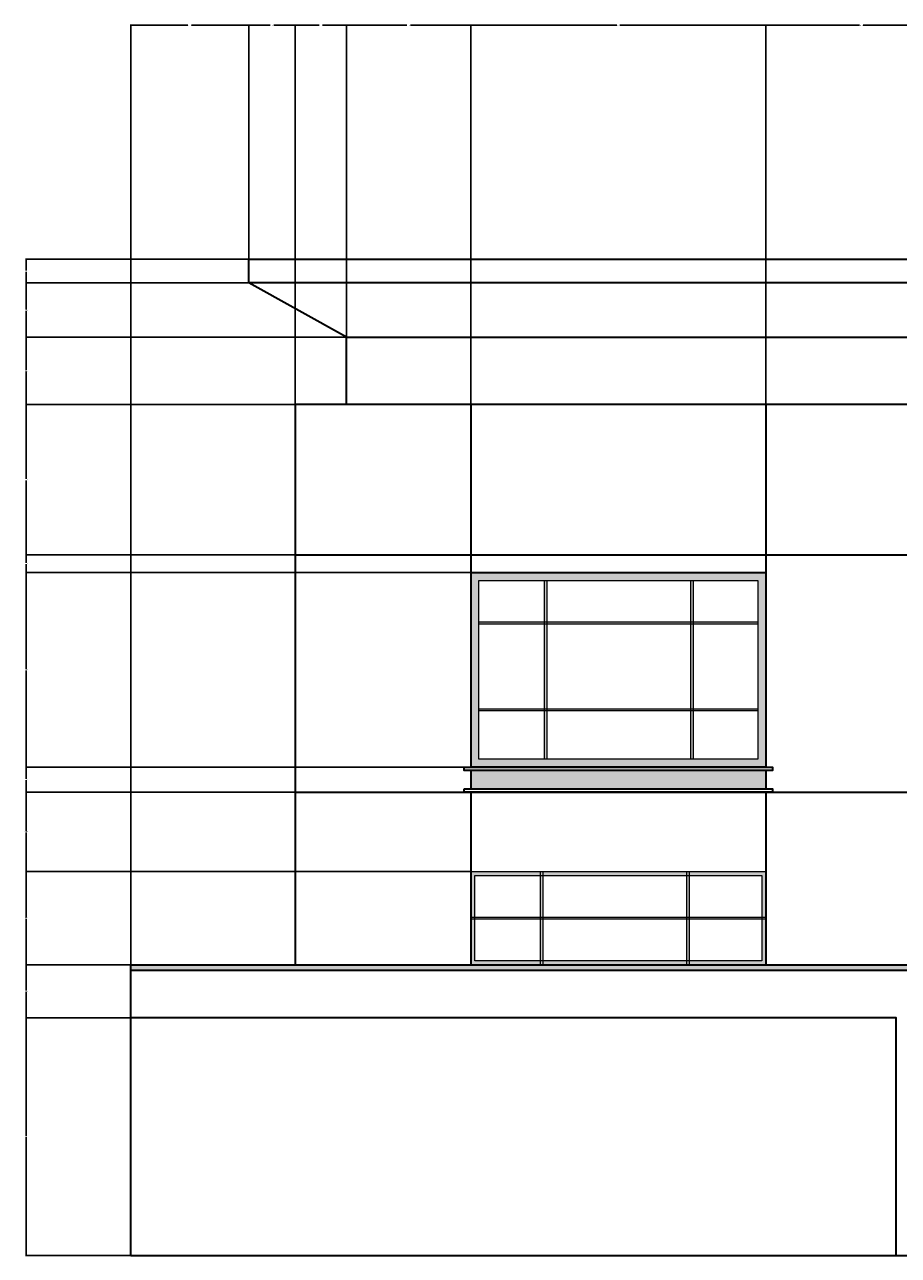
# Model space of a CAD drawing. Units: feet. Extents: x 2651 to 4047, y 949 to 1287.
# Tile 4 of 5: x 3468 to 3689, y 976 to 1287. Entities that reach past the tile are written whole.
import ezdxf

# ---------------------------------------------------------------- set-up
doc = ezdxf.new("R2010")
doc.units = ezdxf.units.FT
for name, color, linetype, lineweight in [('A-ANNO-DIMS', 2, 'Continuous', 18), ('A-ELEV', 7, 'Continuous', 35), ('A-ELEV-PATT', 8, 'Continuous', 13), ('A-GLAZ', 4, 'Continuous', 18)]:
    doc.layers.add(name, color=color, linetype=linetype, lineweight=lineweight)
doc.styles.get("Standard").update_dxf_attribs({"font": 'arial.ttf'})
doc.dimstyles.get("Standard").update_dxf_attribs({"dimtxt": 0.18, "dimasz": 0.18, "dimexe": 0.18, "dimexo": 0.0625, "dimgap": 0.09, "dimtad": 0, "dimtih": 1, "dimtoh": 1, "dimdec": 1, "dimzin": 0, "dimdsep": 46, "dimlunit": 3, "dimtxsty": 'Standard', "dimcen": 0.09, "dimadec": 0, "dimazin": 0, "dimtfac": 1, "dimtdec": 1, "dimtofl": 0, "dimtmove": 0, "dimatfit": 3, "dimfxl": 1, "dimtolj": 1, "dimtzin": 0, "dimarcsym": 0})

# ---------------------------------------------------------------- blocks, each defined once
blk = doc.blocks.new('*D25')
at = {"layer": 'A-ANNO-DIMS', "color": 0, "lineweight": -2, "transparency": 16777216}
for p, q in [((3495.28, 1049.25), (3495.28, 1287.01)), ((3495.46, 1286.83), (3509.71, 1286.83)), ((3524.89, 1286.83), (3510.64, 1286.83)), ((3525.07, 1227.71), (3525.07, 1287.01))]:
    blk.add_line(p, q, dxfattribs=at)
at = {"layer": 'A-ANNO-DIMS', "color": 0, "transparency": 16777216}
for points in [[(3495.46, 1286.86), (3495.46, 1286.8), (3495.28, 1286.83)], [(3524.89, 1286.86), (3524.89, 1286.8), (3525.07, 1286.83)]]:
    blk.add_solid(points, dxfattribs=at)
at = {"layer": 'Defpoints', "color": 0, "transparency": 16777216}
for p in [(3525.07, 1286.83), (3525.07, 1227.65), (3495.28, 1049.19)]:
    blk.add_point(p, dxfattribs=at)
at = {"layer": 'A-ANNO-DIMS', "color": 0, "transparency": 16777216, "insert": (3510.17, 1286.83), "char_height": 0.18, "attachment_point": 5}
blk.add_mtext('\\A1;29.795', dxfattribs=at)
blk = doc.blocks.new('*D26')
at = {"layer": 'A-ANNO-DIMS', "color": 0, "lineweight": -2, "transparency": 16777216}
for p, q in [((3525.07, 1227.71), (3525.07, 1287.01)), ((3525.25, 1286.83), (3530.49, 1286.83)), ((3536.64, 1286.83), (3531.4, 1286.83)), ((3536.82, 1190.93), (3536.82, 1287.01))]:
    blk.add_line(p, q, dxfattribs=at)
at = {"layer": 'A-ANNO-DIMS', "color": 0, "transparency": 16777216}
for points in [[(3525.25, 1286.86), (3525.25, 1286.8), (3525.07, 1286.83)], [(3536.64, 1286.86), (3536.64, 1286.8), (3536.82, 1286.83)]]:
    blk.add_solid(points, dxfattribs=at)
at = {"layer": 'Defpoints', "color": 0, "transparency": 16777216}
for p in [(3536.82, 1286.83), (3525.07, 1227.65), (3536.82, 1190.87)]:
    blk.add_point(p, dxfattribs=at)
at = {"layer": 'A-ANNO-DIMS', "color": 0, "transparency": 16777216, "insert": (3530.95, 1286.83), "char_height": 0.18, "attachment_point": 5}
blk.add_mtext('\\A1;11.753', dxfattribs=at)
blk = doc.blocks.new('*D27')
at = {"layer": 'A-ANNO-DIMS', "color": 0, "lineweight": -2, "transparency": 16777216}
for p, q in [((3536.82, 1190.93), (3536.82, 1287.01)), ((3537, 1286.83), (3542.92, 1286.83)), ((3549.6, 1286.83), (3543.69, 1286.83)), ((3549.78, 1208.02), (3549.78, 1287.01))]:
    blk.add_line(p, q, dxfattribs=at)
at = {"layer": 'A-ANNO-DIMS', "color": 0, "transparency": 16777216}
for points in [[(3537, 1286.86), (3537, 1286.8), (3536.82, 1286.83)], [(3549.6, 1286.86), (3549.6, 1286.8), (3549.78, 1286.83)]]:
    blk.add_solid(points, dxfattribs=at)
at = {"layer": 'Defpoints', "color": 0, "transparency": 16777216}
for p in [(3549.78, 1286.83), (3549.78, 1207.95), (3536.82, 1190.87)]:
    blk.add_point(p, dxfattribs=at)
at = {"layer": 'A-ANNO-DIMS', "color": 0, "transparency": 16777216, "insert": (3543.3, 1286.83), "char_height": 0.18, "attachment_point": 5}
blk.add_mtext('\\A1;12.96', dxfattribs=at)
blk = doc.blocks.new('*D28')
at = {"layer": 'A-ANNO-DIMS', "color": 0, "lineweight": -2, "transparency": 16777216}
for p, q in [((3549.78, 1208.02), (3549.78, 1287.01)), ((3549.96, 1286.83), (3565.05, 1286.83)), ((3581.07, 1286.83), (3565.98, 1286.83)), ((3581.25, 1190.93), (3581.25, 1287.01))]:
    blk.add_line(p, q, dxfattribs=at)
at = {"layer": 'A-ANNO-DIMS', "color": 0, "transparency": 16777216}
for points in [[(3549.96, 1286.86), (3549.96, 1286.8), (3549.78, 1286.83)], [(3581.07, 1286.86), (3581.07, 1286.8), (3581.25, 1286.83)]]:
    blk.add_solid(points, dxfattribs=at)
at = {"layer": 'Defpoints', "color": 0, "transparency": 16777216}
for p in [(3581.25, 1286.83), (3549.78, 1207.95), (3581.25, 1190.87)]:
    blk.add_point(p, dxfattribs=at)
at = {"layer": 'A-ANNO-DIMS', "color": 0, "transparency": 16777216, "insert": (3565.52, 1286.83), "char_height": 0.18, "attachment_point": 5}
blk.add_mtext('\\A1;31.464', dxfattribs=at)
blk = doc.blocks.new('*D29')
at = {"layer": 'A-ANNO-DIMS', "color": 0, "lineweight": -2, "transparency": 16777216}
for p, q in [((3581.25, 1190.93), (3581.25, 1287.01)), ((3581.43, 1286.83), (3618.14, 1286.83)), ((3655.64, 1286.83), (3618.93, 1286.83)), ((3655.82, 1190.93), (3655.82, 1287.01))]:
    blk.add_line(p, q, dxfattribs=at)
at = {"layer": 'A-ANNO-DIMS', "color": 0, "transparency": 16777216}
for points in [[(3581.43, 1286.86), (3581.43, 1286.8), (3581.25, 1286.83)], [(3655.64, 1286.86), (3655.64, 1286.8), (3655.82, 1286.83)]]:
    blk.add_solid(points, dxfattribs=at)
at = {"layer": 'Defpoints', "color": 0, "transparency": 16777216}
for p in [(3655.82, 1286.83), (3581.25, 1190.87), (3655.82, 1190.87)]:
    blk.add_point(p, dxfattribs=at)
at = {"layer": 'A-ANNO-DIMS', "color": 0, "transparency": 16777216, "insert": (3618.53, 1286.83), "char_height": 0.18, "attachment_point": 5}
blk.add_mtext('\\A1;74.57', dxfattribs=at)
blk = doc.blocks.new('*D30')
at = {"layer": 'A-ANNO-DIMS', "color": 0, "lineweight": -2, "transparency": 16777216}
for p, q in [((3655.82, 1190.93), (3655.82, 1287.01)), ((3656, 1286.83), (3679.52, 1286.83)), ((3703.97, 1286.83), (3680.45, 1286.83)), ((3704.15, 1260.39), (3704.15, 1287.01))]:
    blk.add_line(p, q, dxfattribs=at)
at = {"layer": 'A-ANNO-DIMS', "color": 0, "transparency": 16777216}
for points in [[(3656, 1286.86), (3656, 1286.8), (3655.82, 1286.83)], [(3703.97, 1286.86), (3703.97, 1286.8), (3704.15, 1286.83)]]:
    blk.add_solid(points, dxfattribs=at)
at = {"layer": 'Defpoints', "color": 0, "transparency": 16777216}
for p in [(3704.15, 1286.83), (3704.15, 1260.33), (3655.82, 1190.87)]:
    blk.add_point(p, dxfattribs=at)
at = {"layer": 'A-ANNO-DIMS', "color": 0, "transparency": 16777216, "insert": (3679.99, 1286.83), "char_height": 0.18, "attachment_point": 5}
blk.add_mtext('\\A1;48.335', dxfattribs=at)
blk = doc.blocks.new('*D43')
at = {"layer": 'A-ANNO-DIMS', "color": 0, "lineweight": -2, "transparency": 16777216}
for p, q in [((3495.21, 1035.75), (3468.6, 1035.75)), ((3468.78, 1035.57), (3468.78, 1005.88)), ((3468.78, 975.83), (3468.78, 1005.52)), ((3495.21, 975.65), (3468.6, 975.65))]:
    blk.add_line(p, q, dxfattribs=at)
at = {"layer": 'A-ANNO-DIMS', "color": 0, "transparency": 16777216}
for points in [[(3468.75, 1035.57), (3468.81, 1035.57), (3468.78, 1035.75)], [(3468.75, 975.83), (3468.81, 975.83), (3468.78, 975.65)]]:
    blk.add_solid(points, dxfattribs=at)
at = {"layer": 'Defpoints', "color": 0, "transparency": 16777216}
for p in [(3468.78, 1035.75), (3495.28, 1035.75), (3495.28, 975.65)]:
    blk.add_point(p, dxfattribs=at)
at = {"layer": 'A-ANNO-DIMS', "color": 0, "transparency": 16777216, "insert": (3468.78, 1005.7), "char_height": 0.18, "attachment_point": 5}
blk.add_mtext('\\A1;60.1', dxfattribs=at)
blk = doc.blocks.new('*D44')
at = {"layer": 'A-ANNO-DIMS', "color": 0, "lineweight": -2, "transparency": 16777216}
for p, q in [((3536.76, 1049.19), (3468.6, 1049.19)), ((3468.78, 1049.01), (3468.78, 1042.65)), ((3468.78, 1035.93), (3468.78, 1042.29)), ((3495.21, 1035.75), (3468.6, 1035.75))]:
    blk.add_line(p, q, dxfattribs=at)
at = {"layer": 'A-ANNO-DIMS', "color": 0, "transparency": 16777216}
for points in [[(3468.75, 1049.01), (3468.81, 1049.01), (3468.78, 1049.19)], [(3468.75, 1035.93), (3468.81, 1035.93), (3468.78, 1035.75)]]:
    blk.add_solid(points, dxfattribs=at)
at = {"layer": 'Defpoints', "color": 0, "transparency": 16777216}
for p in [(3468.78, 1049.19), (3536.82, 1049.19), (3495.28, 1035.75)]:
    blk.add_point(p, dxfattribs=at)
at = {"layer": 'A-ANNO-DIMS', "color": 0, "transparency": 16777216, "insert": (3468.78, 1042.47), "char_height": 0.18, "attachment_point": 5}
blk.add_mtext('\\A1;13.436', dxfattribs=at)
blk = doc.blocks.new('*D45')
at = {"layer": 'A-ANNO-DIMS', "color": 0, "lineweight": -2, "transparency": 16777216}
for p, q in [((3581.19, 1072.76), (3468.6, 1072.76)), ((3468.78, 1072.58), (3468.78, 1061.15)), ((3468.78, 1049.37), (3468.78, 1060.79)), ((3536.76, 1049.19), (3468.6, 1049.19))]:
    blk.add_line(p, q, dxfattribs=at)
at = {"layer": 'A-ANNO-DIMS', "color": 0, "transparency": 16777216}
for points in [[(3468.75, 1072.58), (3468.81, 1072.58), (3468.78, 1072.76)], [(3468.75, 1049.37), (3468.81, 1049.37), (3468.78, 1049.19)]]:
    blk.add_solid(points, dxfattribs=at)
at = {"layer": 'Defpoints', "color": 0, "transparency": 16777216}
for p in [(3468.78, 1072.76), (3581.25, 1072.76), (3536.82, 1049.19)]:
    blk.add_point(p, dxfattribs=at)
at = {"layer": 'A-ANNO-DIMS', "color": 0, "transparency": 16777216, "insert": (3468.78, 1060.97), "char_height": 0.18, "attachment_point": 5}
blk.add_mtext('\\A1;23.57', dxfattribs=at)
blk = doc.blocks.new('*D46')
at = {"layer": 'A-ANNO-DIMS', "color": 0, "lineweight": -2, "transparency": 16777216}
for p, q in [((3536.76, 1092.85), (3468.6, 1092.85)), ((3468.78, 1092.67), (3468.78, 1082.99)), ((3468.78, 1072.94), (3468.78, 1082.62)), ((3581.19, 1072.76), (3468.6, 1072.76))]:
    blk.add_line(p, q, dxfattribs=at)
at = {"layer": 'A-ANNO-DIMS', "color": 0, "transparency": 16777216}
for points in [[(3468.75, 1092.67), (3468.81, 1092.67), (3468.78, 1092.85)], [(3468.75, 1072.94), (3468.81, 1072.94), (3468.78, 1072.76)]]:
    blk.add_solid(points, dxfattribs=at)
at = {"layer": 'Defpoints', "color": 0, "transparency": 16777216}
for p in [(3468.78, 1092.85), (3536.82, 1092.85), (3581.25, 1072.76)]:
    blk.add_point(p, dxfattribs=at)
at = {"layer": 'A-ANNO-DIMS', "color": 0, "transparency": 16777216, "insert": (3468.78, 1082.81), "char_height": 0.18, "attachment_point": 5}
blk.add_mtext('\\A1;20.096', dxfattribs=at)
blk = doc.blocks.new('*D47')
at = {"layer": 'A-ANNO-DIMS', "color": 0, "lineweight": -2, "transparency": 16777216}
for p, q in [((3581.19, 1099.17), (3468.6, 1099.17)), ((3468.78, 1098.99), (3468.78, 1096.2)), ((3468.78, 1093.03), (3468.78, 1095.83)), ((3536.76, 1092.85), (3468.6, 1092.85))]:
    blk.add_line(p, q, dxfattribs=at)
at = {"layer": 'A-ANNO-DIMS', "color": 0, "transparency": 16777216}
for points in [[(3468.75, 1098.99), (3468.81, 1098.99), (3468.78, 1099.17)], [(3468.75, 1093.03), (3468.81, 1093.03), (3468.78, 1092.85)]]:
    blk.add_solid(points, dxfattribs=at)
at = {"layer": 'Defpoints', "color": 0, "transparency": 16777216}
for p in [(3468.78, 1099.17), (3581.25, 1099.17), (3536.82, 1092.85)]:
    blk.add_point(p, dxfattribs=at)
at = {"layer": 'A-ANNO-DIMS', "color": 0, "transparency": 16777216, "insert": (3468.78, 1096.01), "char_height": 0.18, "attachment_point": 5}
blk.add_mtext('\\A1;6.322', dxfattribs=at)
blk = doc.blocks.new('*D48')
at = {"layer": 'A-ANNO-DIMS', "color": 0, "lineweight": -2, "transparency": 16777216}
for p, q in [((3581.19, 1148.41), (3468.6, 1148.41)), ((3468.78, 1148.23), (3468.78, 1123.98)), ((3468.78, 1099.35), (3468.78, 1123.61)), ((3581.19, 1099.17), (3468.6, 1099.17))]:
    blk.add_line(p, q, dxfattribs=at)
at = {"layer": 'A-ANNO-DIMS', "color": 0, "transparency": 16777216}
for points in [[(3468.75, 1148.23), (3468.81, 1148.23), (3468.78, 1148.41)], [(3468.75, 1099.35), (3468.81, 1099.35), (3468.78, 1099.17)]]:
    blk.add_solid(points, dxfattribs=at)
at = {"layer": 'Defpoints', "color": 0, "transparency": 16777216}
for p in [(3468.78, 1148.41), (3581.25, 1148.41), (3581.25, 1099.17)]:
    blk.add_point(p, dxfattribs=at)
at = {"layer": 'A-ANNO-DIMS', "color": 0, "transparency": 16777216, "insert": (3468.78, 1123.79), "char_height": 0.18, "attachment_point": 5}
blk.add_mtext('\\A1;49.24', dxfattribs=at)
blk = doc.blocks.new('*D49')
at = {"layer": 'A-ANNO-DIMS', "color": 0, "lineweight": -2, "transparency": 16777216}
for p, q in [((3536.76, 1152.91), (3468.6, 1152.91)), ((3468.78, 1152.73), (3468.78, 1150.84)), ((3468.78, 1148.59), (3468.78, 1150.48)), ((3581.19, 1148.41), (3468.6, 1148.41))]:
    blk.add_line(p, q, dxfattribs=at)
at = {"layer": 'A-ANNO-DIMS', "color": 0, "transparency": 16777216}
for points in [[(3468.75, 1152.73), (3468.81, 1152.73), (3468.78, 1152.91)], [(3468.75, 1148.59), (3468.81, 1148.59), (3468.78, 1148.41)]]:
    blk.add_solid(points, dxfattribs=at)
at = {"layer": 'Defpoints', "color": 0, "transparency": 16777216}
for p in [(3468.78, 1152.91), (3536.82, 1152.91), (3581.25, 1148.41)]:
    blk.add_point(p, dxfattribs=at)
at = {"layer": 'A-ANNO-DIMS', "color": 0, "transparency": 16777216, "insert": (3468.78, 1150.66), "char_height": 0.18, "attachment_point": 5}
blk.add_mtext('\\A1;4.493', dxfattribs=at)
blk = doc.blocks.new('*D50')
at = {"layer": 'A-ANNO-DIMS', "color": 0, "lineweight": -2, "transparency": 16777216}
for p, q in [((3536.76, 1190.87), (3468.6, 1190.87)), ((3468.78, 1190.69), (3468.78, 1172.07)), ((3468.78, 1153.09), (3468.78, 1171.71)), ((3536.76, 1152.91), (3468.6, 1152.91))]:
    blk.add_line(p, q, dxfattribs=at)
at = {"layer": 'A-ANNO-DIMS', "color": 0, "transparency": 16777216}
for points in [[(3468.75, 1190.69), (3468.81, 1190.69), (3468.78, 1190.87)], [(3468.75, 1153.09), (3468.81, 1153.09), (3468.78, 1152.91)]]:
    blk.add_solid(points, dxfattribs=at)
at = {"layer": 'Defpoints', "color": 0, "transparency": 16777216}
for p in [(3468.78, 1190.87), (3536.82, 1190.87), (3536.82, 1152.91)]:
    blk.add_point(p, dxfattribs=at)
at = {"layer": 'A-ANNO-DIMS', "color": 0, "transparency": 16777216, "insert": (3468.78, 1171.89), "char_height": 0.18, "attachment_point": 5}
blk.add_mtext('\\A1;37.965', dxfattribs=at)
blk = doc.blocks.new('*D51')
at = {"layer": 'A-ANNO-DIMS', "color": 0, "lineweight": -2, "transparency": 16777216}
for p, q in [((3549.72, 1207.95), (3468.6, 1207.95)), ((3468.78, 1207.77), (3468.78, 1199.59)), ((3468.78, 1191.05), (3468.78, 1199.23)), ((3536.76, 1190.87), (3468.6, 1190.87))]:
    blk.add_line(p, q, dxfattribs=at)
at = {"layer": 'A-ANNO-DIMS', "color": 0, "transparency": 16777216}
for points in [[(3468.75, 1207.77), (3468.81, 1207.77), (3468.78, 1207.95)], [(3468.75, 1191.05), (3468.81, 1191.05), (3468.78, 1190.87)]]:
    blk.add_solid(points, dxfattribs=at)
at = {"layer": 'Defpoints', "color": 0, "transparency": 16777216}
for p in [(3468.78, 1207.95), (3549.78, 1207.95), (3536.82, 1190.87)]:
    blk.add_point(p, dxfattribs=at)
at = {"layer": 'A-ANNO-DIMS', "color": 0, "transparency": 16777216, "insert": (3468.78, 1199.41), "char_height": 0.18, "attachment_point": 5}
blk.add_mtext('\\A1;17.082', dxfattribs=at)
blk = doc.blocks.new('*D52')
at = {"layer": 'A-ANNO-DIMS', "color": 0, "lineweight": -2, "transparency": 16777216}
for p, q in [((3525.01, 1221.65), (3468.6, 1221.65)), ((3468.78, 1221.47), (3468.78, 1214.98)), ((3468.78, 1208.13), (3468.78, 1214.62)), ((3549.72, 1207.95), (3468.6, 1207.95))]:
    blk.add_line(p, q, dxfattribs=at)
at = {"layer": 'A-ANNO-DIMS', "color": 0, "transparency": 16777216}
for points in [[(3468.75, 1221.47), (3468.81, 1221.47), (3468.78, 1221.65)], [(3468.75, 1208.13), (3468.81, 1208.13), (3468.78, 1207.95)]]:
    blk.add_solid(points, dxfattribs=at)
at = {"layer": 'Defpoints', "color": 0, "transparency": 16777216}
for p in [(3468.78, 1221.65), (3525.07, 1221.65), (3549.78, 1207.95)]:
    blk.add_point(p, dxfattribs=at)
at = {"layer": 'A-ANNO-DIMS', "color": 0, "transparency": 16777216, "insert": (3468.78, 1214.8), "char_height": 0.18, "attachment_point": 5}
blk.add_mtext('\\A1;13.696', dxfattribs=at)
blk = doc.blocks.new('*D53')
at = {"layer": 'A-ANNO-DIMS', "color": 0, "lineweight": -2, "transparency": 16777216}
for p, q in [((3525.01, 1227.65), (3468.6, 1227.65)), ((3468.78, 1227.47), (3468.78, 1224.83)), ((3468.78, 1221.83), (3468.78, 1224.47)), ((3525.01, 1221.65), (3468.6, 1221.65))]:
    blk.add_line(p, q, dxfattribs=at)
at = {"layer": 'A-ANNO-DIMS', "color": 0, "transparency": 16777216}
for points in [[(3468.75, 1227.47), (3468.81, 1227.47), (3468.78, 1227.65)], [(3468.75, 1221.83), (3468.81, 1221.83), (3468.78, 1221.65)]]:
    blk.add_solid(points, dxfattribs=at)
at = {"layer": 'Defpoints', "color": 0, "transparency": 16777216}
for p in [(3468.78, 1227.65), (3525.07, 1227.65), (3525.07, 1221.65)]:
    blk.add_point(p, dxfattribs=at)
at = {"layer": 'A-ANNO-DIMS', "color": 0, "transparency": 16777216, "insert": (3468.78, 1224.65), "char_height": 0.18, "attachment_point": 5}
blk.add_mtext('\\A1;6', dxfattribs=at)

msp = doc.modelspace()

# ---------------------------------------------------------------- hatches: boundary and pattern name
at = {"layer": 'A-ELEV-PATT'}
h = msp.add_hatch(color=256, dxfattribs=at)
h.paths.add_polyline_path([(3655.8177, 1148.4143), (3581.2486, 1148.4143), (3581.2486, 1099.175), (3655.8177, 1099.175)])
h.paths.add_polyline_path([(3653.8177, 1146.4143), (3653.8177, 1101.175), (3583.2486, 1101.175), (3583.2486, 1146.4143)], flags=16)
h.paths.add_polyline_path([(3637.4637, 1135.9058), (3637.4637, 1113.3773), (3599.831, 1113.3773), (3599.831, 1135.9058)], flags=0)
h.paths.add_polyline_path([(3636.8563, 1135.3515), (3636.8563, 1113.9316), (3600.4385, 1113.9316), (3600.4385, 1135.3515)], flags=0)
h.paths.add_polyline_path([(3600.4385, 1146.4143), (3599.831, 1146.4143), (3599.831, 1135.9058), (3600.4385, 1135.9058)], flags=0)
h.paths.add_polyline_path([(3599.831, 1135.9058), (3583.2486, 1135.9058), (3583.2486, 1135.3515), (3599.831, 1135.3515)], flags=0)
h.paths.add_polyline_path([(3653.8177, 1135.9058), (3637.4637, 1135.9058), (3637.4637, 1135.3515), (3653.8177, 1135.3515)], flags=0)
h.paths.add_polyline_path([(3637.4637, 1146.4143), (3636.8563, 1146.4143), (3636.8563, 1135.9058), (3637.4637, 1135.9058)], flags=0)
h.paths.add_polyline_path([(3653.8177, 1113.9316), (3637.4637, 1113.9316), (3637.4637, 1113.3773), (3653.8177, 1113.3773)], flags=0)
h.paths.add_polyline_path([(3637.4637, 1113.3773), (3636.8563, 1113.3773), (3636.8563, 1101.175), (3637.4637, 1101.175)], flags=0)
h.paths.add_polyline_path([(3599.831, 1113.9316), (3583.2486, 1113.9316), (3583.2486, 1113.3773), (3599.831, 1113.3773)], flags=0)
h.paths.add_polyline_path([(3600.4385, 1113.3773), (3599.831, 1113.3773), (3599.831, 1101.175), (3600.4385, 1101.175)], flags=0)
h.paths.add_polyline_path([(3599.4385, 1061.2489), (3598.831, 1061.2489), (3598.831, 1060.6946), (3599.4385, 1060.6946)])
h.paths.add_polyline_path([(3599.4385, 1072.7574), (3598.831, 1072.7574), (3598.831, 1061.2489), (3599.4385, 1061.2489)])
h.paths.add_polyline_path([(3655.8177, 1061.2489), (3599.4385, 1061.2489), (3599.4385, 1060.6946), (3655.8177, 1060.6946)])
h.paths.add_polyline_path([(3598.831, 1061.2489), (3581.2486, 1061.2489), (3581.2486, 1060.6946), (3598.831, 1060.6946)])
h.paths.add_polyline_path([(3599.4385, 1060.6946), (3598.831, 1060.6946), (3598.831, 1049.1862), (3599.4385, 1049.1862)])
h.paths.add_polyline_path([(3598.831, 1072.7574), (3581.2486, 1072.7574), (3581.2486, 1061.2489), (3582.2486, 1061.2489), (3582.2486, 1071.7574), (3598.831, 1071.7574)])
h.paths.add_polyline_path([(3655.8177, 1072.7574), (3599.4385, 1072.7574), (3599.4385, 1071.7574), (3654.8177, 1071.7574), (3654.8177, 1061.2489), (3655.8177, 1061.2489)])
h.paths.add_polyline_path([(3655.8177, 1060.6946), (3654.8177, 1060.6946), (3654.8177, 1050.1862), (3599.4385, 1050.1862), (3599.4385, 1049.1862), (3655.8177, 1049.1862)])
h.paths.add_polyline_path([(3582.2486, 1060.6946), (3581.2486, 1060.6946), (3581.2486, 1049.1862), (3598.831, 1049.1862), (3598.831, 1050.1862), (3582.2486, 1050.1862)])
h.paths.add_polyline_path([(3636.4637, 1071.7574), (3635.8563, 1071.7574), (3635.8563, 1061.2489), (3636.4637, 1061.2489)], flags=17)
h.paths.add_polyline_path([(3636.4637, 1060.6946), (3635.8563, 1060.6946), (3635.8563, 1050.1862), (3636.4637, 1050.1862)], flags=17)
h.paths.add_polyline_path([(3700.7838, 1049.1862), (3536.8233, 1049.1862), (3495.2762, 1049.1862), (3495.2762, 1047.7503), (3700.7838, 1047.7503)])
h.paths.add_polyline_path([(3728.7466, 1049.1862), (3715.891, 1049.1862), (3715.891, 1047.7503), (3728.7466, 1047.7503)])
h.paths.add_polyline_path([(3750.1785, 1049.1862), (3737.323, 1049.1862), (3737.323, 1047.7503), (3750.1785, 1047.7503)])
h.paths.add_polyline_path([(3771.6104, 1049.1862), (3758.7549, 1049.1862), (3758.7549, 1047.7503), (3771.6104, 1047.7503)])
h.paths.add_polyline_path([(3803.7115, 1049.1862), (3780.1868, 1049.1862), (3780.1868, 1047.7503), (3803.7115, 1047.7503)])
h.paths.add_polyline_path([(3824.9977, 1077.1763), (3799.3274, 1077.1763), (3799.3274, 1049.1862), (3800.3274, 1049.1862), (3800.3274, 1076.1763), (3823.9977, 1076.1763), (3823.9977, 1038.5677), (3803.7115, 1038.5677), (3803.7115, 1037.5677), (3824.9977, 1037.5677)])
h.paths.add_polyline_path([(3878.6944, 1069.9768), (3865.0283, 1069.9768), (3865.0283, 1058.6821), (3878.6944, 1058.6821)])
h.paths.add_polyline_path([(3877.6944, 1068.9768), (3877.6944, 1059.6821), (3866.0283, 1059.6821), (3866.0283, 1068.9768)], flags=16)
h = msp.add_hatch(color=256, dxfattribs=at)
h.paths.add_polyline_path([(3655.8177, 1098.3392), (3581.2486, 1098.3392), (3581.2486, 1093.6891), (3655.8177, 1093.6891)])
h.paths.add_polyline_path([(4018.604, 1092.8533), (3691.5404, 1092.8533), (3691.5404, 1087.7738), (4018.604, 1087.7738)])

# ---------------------------------------------------------------- linework, layer by layer
at = {"layer": 'A-ELEV'}
for p, q in [((3525.0707, 1227.65), (3762.7135, 1227.65)), ((3525.0707, 1221.65), (3525.0707, 1227.65)), ((3756.7135, 1221.65), (3525.0707, 1221.65)), ((3549.7844, 1207.954), (3525.0707, 1221.65)), ((3549.7844, 1190.8721), (3549.7844, 1207.954)), ((3549.7844, 1207.954), (3756.7135, 1207.954)), ((3581.2486, 1190.8721), (3581.2486, 1099.175)), ((3655.8177, 1190.8721), (3655.8177, 1099.175)), ((3536.8233, 1152.9072), (3704.7437, 1152.9072)), ((3581.2486, 1098.3392), (3581.2486, 1093.6891)), ((3655.8177, 1098.3392), (3655.8177, 1093.6891)), ((3536.8233, 1092.8533), (3704.7437, 1092.8533)), ((3581.2486, 1092.8533), (3581.2486, 1049.1862)), ((3655.8177, 1092.8533), (3655.8177, 1049.1862)), ((3495.2762, 975.65), (3495.2762, 1049.1862)), ((3495.2762, 975.65), (4013.7286, 975.65))]:
    msp.add_line(p, q, dxfattribs=at)
for points in [[(3704.7437, 1095.65), (3704.7437, 1190.8721), (3536.8233, 1190.8721), (3536.8233, 1049.1862), (3704.7437, 1049.1862), (3704.7437, 1084.9772)], [(3581.2486, 1148.4143), (3655.8177, 1148.4143)], [(3655.8177, 1099.175), (3581.2486, 1099.175)], [(3700.7838, 1047.7503), (3495.2762, 1047.7503), (3495.2762, 1049.1862), (3700.7838, 1049.1862)], [(3700.7838, 975.65), (3700.7838, 1047.7503), (3495.2762, 1047.7503)], [(3688.7838, 975.65), (3688.7838, 1035.7503), (3495.2762, 1035.7503)]]:
    msp.add_lwpolyline(points, dxfattribs=at)
for points in [[(3579.5327, 1099.175), (3657.5336, 1099.175), (3657.5336, 1098.3392), (3579.5327, 1098.3392)], [(3579.5327, 1093.6891), (3657.5336, 1093.6891), (3657.5336, 1092.8533), (3579.5327, 1092.8533)]]:
    msp.add_lwpolyline(points, close=True, dxfattribs=at)
at = {"layer": 'A-GLAZ'}
for points in [[(3583.2486, 1146.4143), (3653.8177, 1146.4143), (3653.8177, 1101.175), (3583.2486, 1101.175)], [(3655.8177, 1049.1862), (3581.2486, 1049.1862), (3581.2486, 1072.7574), (3655.8177, 1072.7574)], [(3654.8177, 1050.1862), (3582.2486, 1050.1862), (3582.2486, 1071.7574), (3654.8177, 1071.7574)], [(3598.831, 1072.7574), (3599.4385, 1072.7574), (3599.4385, 1049.1862), (3598.831, 1049.1862)], [(3635.8563, 1072.7574), (3636.4637, 1072.7574), (3636.4637, 1049.1862), (3635.8563, 1049.1862)], [(3581.2486, 1061.2489), (3655.8177, 1061.2489), (3655.8177, 1060.6946), (3581.2486, 1060.6946)]]:
    msp.add_lwpolyline(points, close=True, dxfattribs=at)
for points in [[(3599.831, 1101.175), (3599.831, 1146.4143)], [(3600.4385, 1146.4143), (3600.4385, 1101.175)], [(3636.8563, 1101.175), (3636.8563, 1146.4143)], [(3637.4637, 1146.4143), (3637.4637, 1101.175)], [(3583.2486, 1135.9058), (3653.8177, 1135.9058)], [(3653.8177, 1135.3515), (3583.2486, 1135.3515)], [(3583.2486, 1113.9316), (3653.8177, 1113.9316)], [(3653.8177, 1113.3773), (3583.2486, 1113.3773)]]:
    msp.add_lwpolyline(points, dxfattribs=at)

# ---------------------------------------------------------------- dimensions: what is measured, and where the dimension line sits
at = {"layer": 'A-ANNO-DIMS'}
for base, p1, p2, override, picture, middle in [((3525.07071, 1286.83101), (3495.27616, 1049.18619), (3525.07071, 1227.64997), {"dimdec": 3, "dimlfac": 1, "dimrnd": 0, "dimzin": 0, "dimdsep": 46, "dimlunit": 2}, '*D25', (3510.17343, 1286.83101)), ((3536.8233, 1286.831), (3525.0707, 1227.65), (3536.8233, 1190.8721), {"dimdec": 3, "dimlfac": 1, "dimrnd": 0, "dimzin": 0, "dimdsep": 46, "dimlunit": 2}, '*D26', (3530.947, 1286.831)), ((3549.7844, 1286.831), (3536.8233, 1190.8721), (3549.7844, 1207.954), {"dimdec": 2, "dimlfac": 1, "dimrnd": 0, "dimzin": 0, "dimdsep": 46, "dimlunit": 2}, '*D27', (3543.3038, 1286.831)), ((3581.2486, 1286.831), (3549.7844, 1207.954), (3581.2486, 1190.8721), {"dimdec": 3, "dimlfac": 1, "dimrnd": 0, "dimzin": 0, "dimdsep": 46, "dimlunit": 2}, '*D28', (3565.5165, 1286.831)), ((3655.8177, 1286.831), (3581.2486, 1190.8721), (3655.8177, 1190.8721), {"dimdec": 2, "dimlfac": 1, "dimrnd": 0, "dimzin": 0, "dimdsep": 46, "dimlunit": 2}, '*D29', (3618.5331, 1286.831)), ((3704.1528, 1286.831), (3655.8177, 1190.8721), (3704.1528, 1260.331), {"dimdec": 3, "dimlfac": 1, "dimrnd": 0, "dimzin": 0, "dimdsep": 46, "dimlunit": 2}, '*D30', (3679.9852, 1286.831))]:
    dim = msp.add_linear_dim(base=base, p1=p1, p2=p2, dimstyle='Standard', override=override, dxfattribs=at)
    dim.commit()
    dim.dimension.update_dxf_attribs({"geometry": picture, "text_midpoint": middle})
for base, p1, p2, override, picture, middle in [((3468.7762, 1227.65), (3525.0707, 1221.65), (3525.0707, 1227.65), {"dimdec": 0, "dimlfac": 1, "dimrnd": 0, "dimzin": 0, "dimdsep": 46, "dimlunit": 2}, '*D53', (3468.7762, 1224.65)), ((3468.7762, 1221.65), (3549.7844, 1207.954), (3525.0707, 1221.65), {"dimdec": 3, "dimlfac": 1, "dimrnd": 0, "dimzin": 0, "dimdsep": 46, "dimlunit": 2}, '*D52', (3468.7762, 1214.802)), ((3468.7762, 1207.954), (3536.8233, 1190.8721), (3549.7844, 1207.954), {"dimdec": 3, "dimlfac": 1, "dimrnd": 0, "dimzin": 0, "dimdsep": 46, "dimlunit": 2}, '*D51', (3468.7762, 1199.4131)), ((3468.7762, 1190.8721), (3536.8233, 1152.9072), (3536.8233, 1190.8721), {"dimdec": 3, "dimlfac": 1, "dimrnd": 0, "dimzin": 0, "dimdsep": 46, "dimlunit": 2}, '*D50', (3468.7762, 1171.8897)), ((3468.7762, 1152.9072), (3581.2486, 1148.4143), (3536.8233, 1152.9072), {"dimdec": 3, "dimlfac": 1, "dimrnd": 0, "dimzin": 0, "dimdsep": 46, "dimlunit": 2}, '*D49', (3468.7762, 1150.6608)), ((3468.7762, 1148.4143), (3581.2486, 1099.175), (3581.2486, 1148.4143), {"dimdec": 2, "dimlfac": 1, "dimrnd": 0, "dimzin": 0, "dimdsep": 46, "dimlunit": 2}, '*D48', (3468.7762, 1123.7946)), ((3468.7762, 1099.175), (3536.8233, 1092.8533), (3581.2486, 1099.175), {"dimdec": 3, "dimlfac": 1, "dimrnd": 0, "dimzin": 0, "dimdsep": 46, "dimlunit": 2}, '*D47', (3468.7762, 1096.0141)), ((3468.7762, 1092.8533), (3581.2486, 1072.7574), (3536.8233, 1092.8533), {"dimdec": 3, "dimlfac": 1, "dimrnd": 0, "dimzin": 0, "dimdsep": 46, "dimlunit": 2}, '*D46', (3468.7762, 1082.8053)), ((3468.7762, 1072.7574), (3536.8233, 1049.1862), (3581.2486, 1072.7574), {"dimdec": 2, "dimlfac": 1, "dimrnd": 0, "dimzin": 0, "dimdsep": 46, "dimlunit": 2}, '*D45', (3468.7762, 1060.9718)), ((3468.7762, 1049.1862), (3495.2762, 1035.7503), (3536.8233, 1049.1862), {"dimdec": 3, "dimlfac": 1, "dimrnd": 0, "dimzin": 0, "dimdsep": 46, "dimlunit": 2}, '*D44', (3468.7762, 1042.4682)), ((3468.7762, 1035.7503), (3495.2762, 975.65), (3495.2762, 1035.7503), {"dimdec": 1, "dimlfac": 1, "dimrnd": 0, "dimzin": 0, "dimdsep": 46, "dimlunit": 2}, '*D43', (3468.7762, 1005.7001))]:
    dim = msp.add_linear_dim(base=base, p1=p1, p2=p2, angle=90, dimstyle='Standard', override=override, dxfattribs=at)
    dim.commit()
    dim.dimension.update_dxf_attribs({"geometry": picture, "text_midpoint": middle})

doc.saveas('drawing.dxf')
